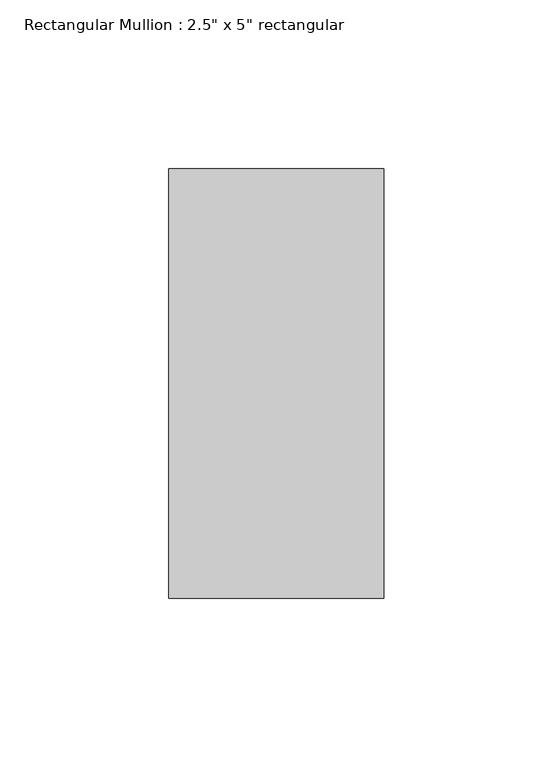
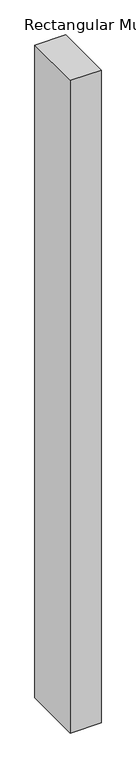
"""IFC4 building model written with IfcOpenShell, lengths in millimetres: member geometry."""

from ifc_helpers import new_model, si_unit, frame, origin, place, context, project, spatial, polyline, outline, extrude, source, transform, mapped, element, save


def member_3473b942(model_context):
    return source(origin(), model_context, "Body", "SweptSolid", [
        extrude(outline(polyline([(0.0, 63.5), (0.0, -63.5), (-63.5, -63.5), (-63.5, 63.5), (0.0, 63.5)])), frame((0.0, 0.0, -1428.7500001), z_axis=(0.0, 0.0, 1.0), x_axis=(1.0, 0.0, 0.0)), (0.0, 0.0, 1.0), 1428.7500001),
    ])


if __name__ == "__main__":
    model = new_model("IFC4")
    model_context = context("Model", 3, world=origin())
    ifc_project = project(units=[si_unit("LENGTHUNIT", "METRE", prefix="MILLI")], contexts=[model_context])
    site = spatial("IfcSite", under=ifc_project)
    building = spatial("IfcBuilding", under=site)
    placement = place(None, origin())
    member_shape = member_3473b942(model_context)
    element("IfcMember", 1, ObjectType="Rectangular Mullion : 2.5\" x 5\" rectangular", at=placement, inside=building, context=model_context, shape_type="MappedRepresentation", body=[
        mapped(member_shape, transform((0.0, 0.0, 0.0), x_axis=(1.0, 0.0, 0.0), y_axis=(0.0, 1.0, 0.0), z_axis=(0.0, 0.0, 1.0))),
    ])
    save(model, "model.ifc")

# Revit data of these elements
# Type "Rectangular Mullion : 2.5\" x 5\" rectangular"
#   built-in parameter 1007304 = 0.416667 (stored number, unit not read)
#   built-in parameter 1007301 = 0.104167 (stored number, unit not read)
#   built-in parameter 1007300 = 0.104167 (stored number, unit not read)
# Element 1 (IfcMember, "Rectangular Mullion : 2.5\" x 5\" rectangular")
#   Materials on its faces: "BLACK COLOUR"
# Materials
#   "BLACK COLOUR": class "Generic", colour RGB 120 120 120, transparency 0, Cost = 0
